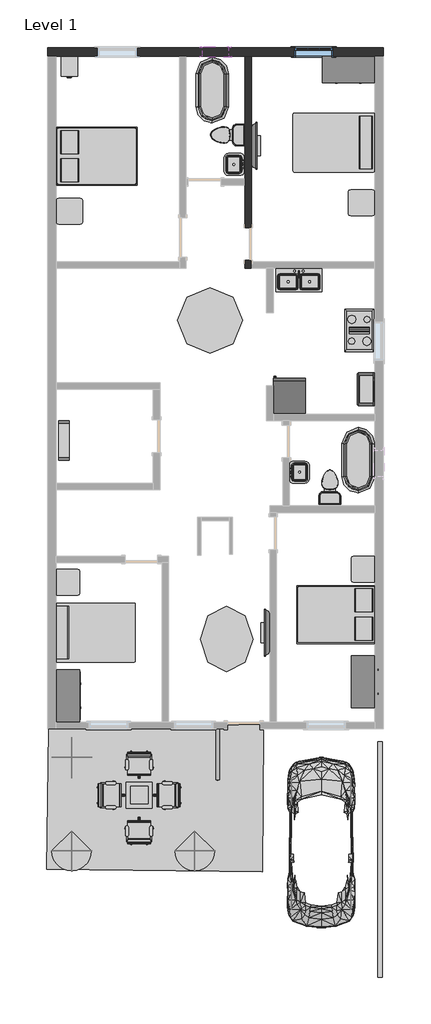
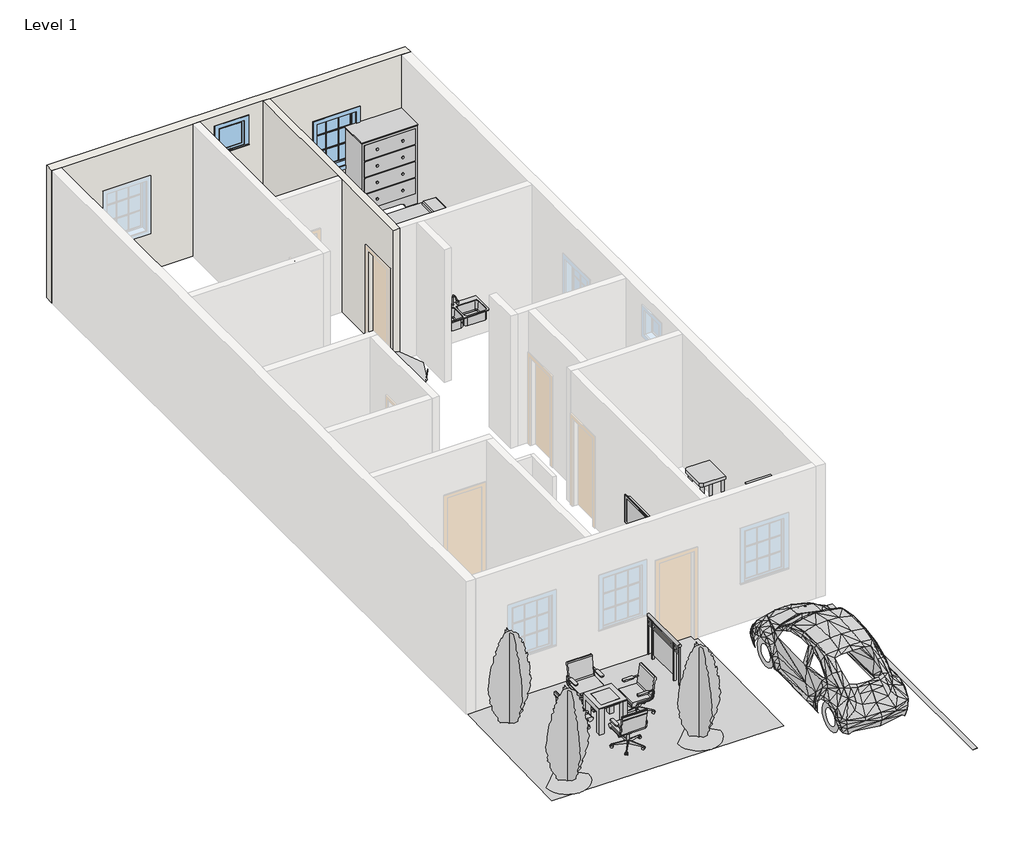
# One storey, part 2 of 2: 22 furniture elements, 7 flow terminals, 6 proxies, 3 geographic elements, 2 walls, 2 windows, 1 railing.
"""IFC4 building model written with IfcOpenShell, lengths in millimetres."""

from ifc_helpers import new_model, si_unit, point, frame, origin, origin_with_axes, place, context, project, spatial, polyline, ellipse_curve, trimmed, outline, extrude, faceted_brep, triangles, transform, mapped, element, save
from ifc_brep_helpers import plane_surface, extruded_surface, advanced_brep
from components import proxy_bb1e6e30, proxy_8a8d5ab2, parking_space_9_x_18_90_deg_b8b21359, rpc_beetle_rpc_beetle_3ce7ba48, proxy_a13a33b2, flow_terminal_a53be723, flow_terminal_62a433f7, toilet_domestic_3d_toilet_domestic_3d_f7549cf7, toilet_domestic_3d_toilet_domestic_3d_183bbd19, flow_terminal_b374fae2, furniture_c8abb964, furniture_0253826f, furniture_552c1472, chair_task_arms_chair_task_arms_fa5a08ef, furniture_9fa109b2, furniture_417d203a, furniture_7a3aaa4f, furniture_b5c51a22, furniture_bbcc68ce, furniture_743965d2, furniture_bcf351fa, rpc_tree_conifer_chinese_juniper_7_1b9786cd, window_29c06734, window_e41d21a6

model = new_model("IFC4")

# Units and contexts
model_context = context("Model", 3, world=origin())
ifc_project = project(units=[si_unit("LENGTHUNIT", "METRE", prefix="MILLI")], contexts=[model_context])

# Site, building, storey
site = spatial("IfcSite", under=ifc_project)
building = spatial("IfcBuilding", under=site)
storey = spatial("IfcBuildingStorey", under=building, Name="Level 1", Elevation=0.0)

# Proxies
placement = place(None, origin())
element("IfcBuildingElementProxy", 1, Name="Building Element Proxy", at=placement, inside=storey, context=model_context, shape_type="Tessellation", body=[
    triangles([(-16242.6911224, -4685.5730095, 0.0), (-16293.4903473, -7924.0733002, 0.0), (-11264.2903473, -7980.080928, 0.0), (-11238.8907349, -4679.2231064, 0.0), (-11238.8907349, -4653.8232033, 0.0), (-11315.0907349, -4552.2230095, 0.0), (-16242.6911224, -4672.8732033, 0.0)], [[2, 1, 7], [1, 2, 3], [7, 1, 6], [4, 6, 1], [5, 6, 4], [4, 1, 3]], closed=False),
])
proxy_shape = proxy_bb1e6e30(model_context)
element("IfcBuildingElementProxy", 2, Name="Cook Top-4 Unit : 36\" x 20\"", ObjectType="Cook Top-4 Unit : 36\" x 20\"", at=placement, inside=storey, context=model_context, shape_type="MappedRepresentation", body=[
    mapped(proxy_shape, transform((-9003.6905738, 4617.1768478, 0.0), x_axis=(0.0, 1.0000000000000009, 0.0), y_axis=(-1.0000000000000009, 0.0, 0.0), z_axis=(0.0, 0.0, 1.0))),
])
proxy_2_shape = proxy_8a8d5ab2(model_context)
element("IfcBuildingElementProxy", 3, Name="Microwave : 30\" x 16\" x 18\"", ObjectType="Microwave : 30\" x 16\" x 18\"", at=placement, inside=storey, context=model_context, shape_type="MappedRepresentation", body=[
    mapped(proxy_2_shape, transform((-9204.3710796, 2745.2839704, 0.0), x_axis=(0.0, 1.0000000000000002, 0.0), y_axis=(-1.0000000000000002, 0.0, 0.0), z_axis=(0.0, 0.0, 1.0))),
])
parking_space_9_x_18_90_deg_shape = parking_space_9_x_18_90_deg_b8b21359(model_context)
element("IfcBuildingElementProxy", 4, Name="Parking Space : 9' x 18' - 90 deg", ObjectType="Parking Space : 9' x 18' - 90 deg", at=placement, inside=storey, context=model_context, shape_type="MappedRepresentation", body=[
    mapped(parking_space_9_x_18_90_deg_shape, transform((-8521.0905738, -10445.0231522, 0.0), x_axis=(-1.0, 0.0, 0.0), y_axis=(0.0, -1.0, 0.0), z_axis=(0.0, 0.0, 1.0))),
])
rpc_beetle_rpc_beetle_shape = rpc_beetle_rpc_beetle_3ce7ba48(model_context)
element("IfcBuildingElementProxy", 5, Name="RPC Beetle : RPC Beetle", ObjectType="RPC Beetle : RPC Beetle", at=placement, inside=storey, context=model_context, shape_type="MappedRepresentation", body=[
    mapped(rpc_beetle_rpc_beetle_shape, transform((-9892.6905738, -8540.0231522, 0.0), x_axis=(1.0, 0.0, 0.0), y_axis=(0.0, 1.0, 0.0), z_axis=(0.0, 0.0, 1.0))),
])
proxy_3_shape = proxy_a13a33b2(model_context)
element("IfcBuildingElementProxy", 6, Name="Refrigerator : 30\" x 32\" RH", ObjectType="Refrigerator : 30\" x 32\" RH", at=placement, inside=storey, context=model_context, shape_type="MappedRepresentation", body=[
    mapped(proxy_3_shape, transform((-10637.2280738, 3079.2778763, 0.0), x_axis=(-1.0000000000000004, 0.0, 0.0), y_axis=(0.0, -1.0000000000000004, 0.0), z_axis=(0.0, 0.0, 1.0))),
])

# Flow terminals
flow_terminal_shape = flow_terminal_a53be723(model_context)
element("IfcFlowTerminal", 7, ObjectType="Sink Kitchen-Double : 42\" x 21\"", at=placement, inside=storey, context=model_context, shape_type="MappedRepresentation", body=[
    mapped(flow_terminal_shape, transform((-10429.0798144, 5783.2314467, 0.0), x_axis=(1.0, 0.0, 0.0), y_axis=(0.0, 1.0, 0.0), z_axis=(0.0, 0.0, 1.0))),
])
flow_terminal_2_shape = flow_terminal_62a433f7(model_context)
element("IfcFlowTerminal", 8, ObjectType="Sink Vanity-Square : 20\" x 18\"", at=placement, inside=storey, context=model_context, shape_type="MappedRepresentation", body=[
    mapped(flow_terminal_2_shape, transform((-11876.2359749, 8493.6660883, 304.8), x_axis=(0.0, -1.0000000000000004, 0.0), y_axis=(1.0000000000000004, 0.0, 0.0), z_axis=(0.0, 0.0, 1.0))),
])
element("IfcFlowTerminal", 9, ObjectType="Sink Vanity-Square : 20\" x 18\"", at=placement, inside=storey, context=model_context, shape_type="MappedRepresentation", body=[
    mapped(flow_terminal_2_shape, transform((-10449.1451727, 1299.4876072, 304.8), x_axis=(0.0, 1.0, 0.0), y_axis=(-1.0, 0.0, 0.0), z_axis=(0.0, 0.0, 1.0))),
])
toilet_domestic_3d_toilet_domestic_3d_shape = toilet_domestic_3d_toilet_domestic_3d_f7549cf7(model_context)
toilet_domestic_3d_toilet_domestic_3d_2_shape = toilet_domestic_3d_toilet_domestic_3d_183bbd19(model_context)
element("IfcFlowTerminal", 10, ObjectType="Toilet-Domestic-3D : Toilet-Domestic-3D", at=placement, inside=storey, context=model_context, shape_type="MappedRepresentation", body=[
    mapped(toilet_domestic_3d_toilet_domestic_3d_shape, transform((-12165.3866012, 9163.7768478, 0.0), x_axis=(0.0, -1.0000000000000002, 0.0), y_axis=(1.0000000000000002, 0.0, 0.0), z_axis=(0.0, 0.0, 1.0))),
    mapped(toilet_domestic_3d_toilet_domestic_3d_2_shape, transform((-12165.3866012, 9163.7768478, 0.0), x_axis=(0.0, -1.0000000000000002, 0.0), y_axis=(1.0000000000000002, 0.0, 0.0), z_axis=(0.0, 0.0, 1.0))),
])
element("IfcFlowTerminal", 11, ObjectType="Toilet-Domestic-3D : Toilet-Domestic-3D", at=placement, inside=storey, context=model_context, shape_type="MappedRepresentation", body=[
    mapped(toilet_domestic_3d_toilet_domestic_3d_shape, transform((-9689.4905738, 1061.1768478, 0.0), x_axis=(-0.9999999999999998, 0.0, 0.0), y_axis=(0.0, -0.9999999999999998, 0.0), z_axis=(0.0, 0.0, 1.0))),
    mapped(toilet_domestic_3d_toilet_domestic_3d_2_shape, transform((-9689.4905738, 1061.1768478, 0.0), x_axis=(-0.9999999999999998, 0.0, 0.0), y_axis=(0.0, -0.9999999999999998, 0.0), z_axis=(0.0, 0.0, 1.0))),
])
flow_terminal_3_shape = flow_terminal_b374fae2(model_context)
element("IfcFlowTerminal", 12, ObjectType="Tub-Free Standing-3D : 30\" x 60\"", at=placement, inside=storey, context=model_context, shape_type="MappedRepresentation", body=[
    mapped(flow_terminal_3_shape, transform((-12432.6905738, 10205.1768478, 0.0), x_axis=(1.0, 0.0, 0.0), y_axis=(0.0, 1.0, 0.0), z_axis=(0.0, 0.0, 1.0))),
])
element("IfcFlowTerminal", 13, ObjectType="Tub-Free Standing-3D : 30\" x 60\"", at=placement, inside=storey, context=model_context, shape_type="MappedRepresentation", body=[
    mapped(flow_terminal_3_shape, transform((-9029.0905738, 1594.5768478, 0.0), x_axis=(1.0, 0.0, 0.0), y_axis=(0.0, 1.0, 0.0), z_axis=(0.0, 0.0, 1.0))),
])

# Furniture
furniture_shape = furniture_c8abb964(model_context)
element("IfcFurniture", 14, ObjectType="Bed-Box : Double 53\" x 74\"", at=placement, inside=storey, context=model_context, shape_type="MappedRepresentation", body=[
    mapped(furniture_shape, transform((-15359.520082, 8329.3243888, 0.0), x_axis=(0.0, 1.0, 0.0), y_axis=(-1.0, 0.0, 0.0), z_axis=(0.0, 0.0, 1.0))),
])
element("IfcFurniture", 15, ObjectType="Bed-Box : Double 53\" x 74\"", at=placement, inside=storey, context=model_context, shape_type="MappedRepresentation", body=[
    mapped(furniture_shape, transform((-9289.9610656, -1660.3706932, 0.0), x_axis=(0.0, -1.0, 0.0), y_axis=(1.0, 0.0, 0.0), z_axis=(0.0, 0.0, 1.0))),
])
furniture_2_shape = furniture_0253826f(model_context)
element("IfcFurniture", 16, ObjectType="Bed-Standard.0001 : Double 54\" x 75\"", at=placement, inside=storey, context=model_context, shape_type="MappedRepresentation", body=[
    mapped(furniture_2_shape, transform((-9554.9954918, 9257.4653724, 0.0), x_axis=(0.0, -1.0000000000000002, 0.0), y_axis=(1.0000000000000002, 0.0, 0.0), z_axis=(0.0, 0.0, 1.0))),
])
element("IfcFurniture", 17, ObjectType="Bed-Standard.0001 : Double 54\" x 75\"", at=placement, inside=storey, context=model_context, shape_type="MappedRepresentation", body=[
    mapped(furniture_2_shape, transform((-15221.4856558, -2690.1116768, 0.0), x_axis=(0.0, 1.0, 0.0), y_axis=(-1.0, 0.0, 0.0), z_axis=(0.0, 0.0, 1.0))),
])
furniture_3_shape = furniture_552c1472(model_context)
element("IfcFurniture", 18, ObjectType="Cabinet-File 3 Drawer.0001 : 15\" x 18\"", at=placement, inside=storey, context=model_context, shape_type="MappedRepresentation", body=[
    mapped(furniture_3_shape, transform((-15632.1941268, 10906.1111479, 0.0), x_axis=(1.0, 0.0, 0.0), y_axis=(0.0, 1.0, 0.0), z_axis=(0.0, 0.0, 1.0))),
])
chair_task_arms_chair_task_arms_shape = chair_task_arms_chair_task_arms_fa5a08ef(model_context)
element("IfcFurniture", 19, ObjectType="Chair-Task Arms : Chair-Task Arms", at=placement, inside=storey, context=model_context, shape_type="MappedRepresentation", body=[
    mapped(chair_task_arms_chair_task_arms_shape, transform((-13993.4997541, -5447.6772506, 0.0), x_axis=(-1.0000000000000004, 0.0, 0.0), y_axis=(0.0, -1.0000000000000004, 0.0), z_axis=(0.0, 0.0, 1.0))),
])
element("IfcFurniture", 20, ObjectType="Chair-Task Arms : Chair-Task Arms", at=placement, inside=storey, context=model_context, shape_type="MappedRepresentation", body=[
    mapped(chair_task_arms_chair_task_arms_shape, transform((-14839.2364754, -6062.2323326, 0.0), x_axis=(0.0, -1.0000000000000007, 0.0), y_axis=(1.0000000000000007, 0.0, 0.0), z_axis=(0.0, 0.0, 1.0))),
])
element("IfcFurniture", 21, ObjectType="Chair-Task Arms : Chair-Task Arms", at=placement, inside=storey, context=model_context, shape_type="MappedRepresentation", body=[
    mapped(chair_task_arms_chair_task_arms_shape, transform((-14275.4813935, -7085.7690539, 0.0), x_axis=(1.0, 0.0, 0.0), y_axis=(0.0, 1.0, 0.0), z_axis=(0.0, 0.0, 1.0))),
])
element("IfcFurniture", 22, ObjectType="Chair-Task Arms : Chair-Task Arms", at=placement, inside=storey, context=model_context, shape_type="MappedRepresentation", body=[
    mapped(chair_task_arms_chair_task_arms_shape, transform((-13429.7446722, -6344.2139719, 0.0), x_axis=(0.0, 1.0000000000000002, 0.0), y_axis=(-1.0000000000000002, 0.0, 0.0), z_axis=(0.0, 0.0, 1.0))),
])
furniture_4_shape = furniture_9fa109b2(model_context)
element("IfcFurniture", 23, ObjectType="Dresser : 48\" x 72\" x 24\"", at=placement, inside=storey, context=model_context, shape_type="MappedRepresentation", body=[
    mapped(furniture_4_shape, transform((-8988.497314, 11050.9398019, 0.0), x_axis=(1.0, 0.0, 0.0), y_axis=(0.0, 1.0, 0.0), z_axis=(0.0, 0.0, 1.0))),
])
element("IfcFurniture", 24, ObjectType="Dresser : 48\" x 72\" x 24\"", at=placement, inside=storey, context=model_context, shape_type="MappedRepresentation", body=[
    mapped(furniture_4_shape, transform((-9252.5535279, -3292.4298924, 0.0), x_axis=(0.0, 1.0, 0.0), y_axis=(-1.0, 0.0, 0.0), z_axis=(0.0, 0.0, 1.0))),
])
element("IfcFurniture", 25, ObjectType="Dresser : 48\" x 72\" x 24\"", at=placement, inside=storey, context=model_context, shape_type="MappedRepresentation", body=[
    mapped(furniture_4_shape, transform((-16186.7535279, -3622.6298924, 0.0), x_axis=(0.0, 1.0, 0.0), y_axis=(-1.0, 0.0, 0.0), z_axis=(0.0, 0.0, 1.0))),
])
furniture_5_shape = furniture_417d203a(model_context)
element("IfcFurniture", 26, ObjectType="Shelving : 36\" x 10\" x 72\"", at=placement, inside=storey, context=model_context, shape_type="MappedRepresentation", body=[
    mapped(furniture_5_shape, transform((-16191.8905738, 2051.7768478, 0.0), x_axis=(0.0, 1.0000000000000002, 0.0), y_axis=(-1.0000000000000002, 0.0, 0.0), z_axis=(0.0, 0.0, 1.0))),
])
furniture_6_shape = furniture_7a3aaa4f(model_context)
element("IfcFurniture", 27, ObjectType="TV - Flat Screen : 42\"", at=placement, inside=storey, context=model_context, shape_type="MappedRepresentation", body=[
    mapped(furniture_6_shape, transform((-11459.7519502, 8913.7213619, 914.4), x_axis=(0.0, 1.0, 0.0), y_axis=(-1.0, 0.0, 0.0), z_axis=(0.0, 0.0, 1.0))),
])
element("IfcFurniture", 28, ObjectType="TV - Flat Screen : 42\"", at=placement, inside=storey, context=model_context, shape_type="MappedRepresentation", body=[
    mapped(furniture_6_shape, transform((-11145.0291975, -2422.5676664, 914.4), x_axis=(0.0, -1.0000000000000004, 0.0), y_axis=(1.0000000000000004, 0.0, 0.0), z_axis=(0.0, 0.0, 1.0))),
])
furniture_7_shape = furniture_b5c51a22(model_context)
element("IfcFurniture", 29, ObjectType="Table-Coffee : 24\" x 24\" x 24\"", at=placement, inside=storey, context=model_context, shape_type="MappedRepresentation", body=[
    mapped(furniture_7_shape, transform((-14152.7563405, -6298.43423, 0.0), x_axis=(1.0, 0.0, 0.0), y_axis=(0.0, 1.0, 0.0), z_axis=(0.0, 0.0, 1.0))),
])
furniture_8_shape = furniture_bbcc68ce(model_context)
element("IfcFurniture", 30, ObjectType="Table-Dining Round w Chairs : 60\" Diameter", at=placement, inside=storey, context=model_context, shape_type="MappedRepresentation", body=[
    mapped(furniture_8_shape, transform((-12587.172541, 5030.6555363, 0.0), x_axis=(1.0, 0.0, 0.0), y_axis=(0.0, 1.0, 0.0), z_axis=(0.0, 0.0, 1.0))),
])
furniture_9_shape = furniture_743965d2(model_context)
element("IfcFurniture", 31, ObjectType="Table-Ellipse : 60\" x 48\"", at=placement, inside=storey, context=model_context, shape_type="MappedRepresentation", body=[
    mapped(furniture_9_shape, transform((-12097.4549283, -2571.0231522, 0.0), x_axis=(0.0, 1.0000000000000002, 0.0), y_axis=(-1.0000000000000002, 0.0, 0.0), z_axis=(0.0, 0.0, 1.0))),
])
furniture_10_shape = furniture_bcf351fa(model_context)
element("IfcFurniture", 32, ObjectType="Table-End : 24\" x 24\"", at=placement, inside=storey, context=model_context, shape_type="MappedRepresentation", body=[
    mapped(furniture_10_shape, transform((-16068.6242041, 7233.3768478, 0.0), x_axis=(1.0, 0.0, 0.0), y_axis=(0.0, 1.0, 0.0), z_axis=(0.0, 0.0, 1.0))),
])
element("IfcFurniture", 33, ObjectType="Table-End : 24\" x 24\"", at=placement, inside=storey, context=model_context, shape_type="MappedRepresentation", body=[
    mapped(furniture_10_shape, transform((-9261.4242041, 7436.5768478, 0.0), x_axis=(1.0, 0.0, 0.0), y_axis=(0.0, 1.0, 0.0), z_axis=(0.0, 0.0, 1.0))),
])
element("IfcFurniture", 34, ObjectType="Table-End : 24\" x 24\"", at=placement, inside=storey, context=model_context, shape_type="MappedRepresentation", body=[
    mapped(furniture_10_shape, transform((-9197.9242041, -1097.8231522, 0.0), x_axis=(1.0, 0.0, 0.0), y_axis=(0.0, 1.0, 0.0), z_axis=(0.0, 0.0, 1.0))),
])
element("IfcFurniture", 35, ObjectType="Table-End : 24\" x 24\"", at=placement, inside=storey, context=model_context, shape_type="MappedRepresentation", body=[
    mapped(furniture_10_shape, transform((-16132.1242041, -1402.6231522, 0.0), x_axis=(1.0, 0.0, 0.0), y_axis=(0.0, 1.0, 0.0), z_axis=(0.0, 0.0, 1.0))),
])

# Geographic elements
rpc_tree_conifer_chinese_juniper_7_shape = rpc_tree_conifer_chinese_juniper_7_1b9786cd(model_context)
element("IfcGeographicElement", 36, ObjectType="RPC Tree - Conifer : Chinese Juniper - 7'", at=placement, inside=storey, context=model_context, shape_type="MappedRepresentation", body=[
    mapped(rpc_tree_conifer_chinese_juniper_7_shape, transform((-15709.4872449, -5314.2231522, 0.0), x_axis=(1.0, 0.0, 0.0), y_axis=(0.0, 1.0, 0.0), z_axis=(0.0, 0.0, 1.0))),
])
element("IfcGeographicElement", 37, ObjectType="RPC Tree - Conifer : Chinese Juniper - 7'", at=placement, inside=storey, context=model_context, shape_type="MappedRepresentation", body=[
    mapped(rpc_tree_conifer_chinese_juniper_7_shape, transform((-15709.4872449, -7498.6231522, 0.0), x_axis=(1.0, 0.0, 0.0), y_axis=(0.0, 1.0, 0.0), z_axis=(0.0, 0.0, 1.0))),
])
element("IfcGeographicElement", 38, ObjectType="RPC Tree - Conifer : Chinese Juniper - 7'", at=placement, inside=storey, context=model_context, shape_type="MappedRepresentation", body=[
    mapped(rpc_tree_conifer_chinese_juniper_7_shape, transform((-12839.2872449, -7498.6231522, 0.0), x_axis=(1.0, 0.0, 0.0), y_axis=(0.0, 1.0, 0.0), z_axis=(0.0, 0.0, 1.0))),
])

# Railing
element("IfcRailing", 39, ObjectType="Glass Panel - Bottom Fill", at=placement, inside=storey, context=model_context, shape_type="SolidModel", body=[
    advanced_brep(
    [(-12267.5905738, -4653.8231522, 914.4), (-12343.7905738, -4653.8231522, 914.4), (-12267.5905738, -5847.6231522, 914.4), (-12343.7905738, -5847.6231522, 914.4)],
    [
        (0, 1, ellipse_curve(frame((-12305.6905738, -4653.8231522, 914.4), z_axis=(0.0, 1.0, 0.0), x_axis=(-1.0, 0.0, 0.0)), 38.1, 28.575)),
        (1, 0, ellipse_curve(frame((-12305.6905738, -4653.8231522, 914.4), z_axis=(0.0, 1.0, 0.0), x_axis=(-1.0, 0.0, 0.0)), 38.1, 28.575)),
        (2, 3, ellipse_curve(frame((-12305.6905738, -5847.6231522, 914.4), z_axis=(0.0, -1.0, 0.0), x_axis=(-1.0, 0.0, 0.0)), 38.1, 28.575)),
        (3, 2, ellipse_curve(frame((-12305.6905738, -5847.6231522, 914.4), z_axis=(0.0, -1.0, 0.0), x_axis=(-1.0, 0.0, 0.0)), 38.1, 28.575)),
        (0, 2),
        (3, 1),
    ],
    [
        plane_surface(frame((-12305.6905738, -4653.8231522, 914.4), z_axis=(0.0, 1.0, 0.0), x_axis=(0.0, 0.0, -1.0))),
        plane_surface(frame((-12305.6905738, -5847.6231522, 914.4), z_axis=(0.0, -1.0, 0.0), x_axis=(0.0, 0.0, -1.0))),
        extruded_surface(trimmed(ellipse_curve(frame((-12305.6905738, -5847.6231522, 914.4), z_axis=(0.0, 1.0, 0.0), x_axis=(-1.0, 0.0, 0.0)), 38.1, 28.575), [point((-12267.5905738, -5847.6231522, 914.4))], [point((-12343.7905738, -5847.6231522, 914.4))], True, "CARTESIAN"), (0.0, 1193.8000000000002, 0.0), 1193.8000000000002),
        extruded_surface(trimmed(ellipse_curve(frame((-12305.6905738, -5847.6231522, 914.4), z_axis=(0.0, 1.0, 0.0), x_axis=(-1.0, 0.0, 0.0)), 38.1, 28.575), [point((-12343.7905738, -5847.6231522, 914.4))], [point((-12267.5905738, -5847.6231522, 914.4))], True, "CARTESIAN"), (0.0, 1193.8000000000002, 0.0), 1193.8000000000002),
    ],
    [
        (0, [[1, 2]]),
        (1, [[3, 4]]),
        (2, [[-1, 5, -4, 6]]),
        (3, [[-2, -6, -3, -5]]),
    ],
),
    extrude(outline(polyline([(-12318.3905738, -4653.8231522), (-12292.9905738, -4653.8231522), (-12292.9905738, -5847.6231522), (-12318.3905738, -5847.6231522), (-12318.3905738, -4653.8231522)])), frame((0.0, 0.0, 800.1), z_axis=(0.0, 0.0, 1.0), x_axis=(1.0, 0.0, 0.0)), (0.0, 0.0, 1.0), 25.4),
    extrude(outline(polyline([(-12318.3905738, -4653.8231522), (-12292.9905738, -4653.8231522), (-12292.9905738, -5847.6231522), (-12318.3905738, -5847.6231522), (-12318.3905738, -4653.8231522)])), frame((0.0, 0.0, 698.5), z_axis=(0.0, 0.0, 1.0), x_axis=(1.0, 0.0, 0.0)), (0.0, 0.0, 1.0), 25.4),
    extrude(outline(polyline([(-12331.0905738, -5650.7731522), (-12280.2905738, -5650.7731522), (-12280.2905738, -5663.4731522), (-12331.0905738, -5663.4731522), (-12331.0905738, -5650.7731522)])), origin_with_axes(), (0.0, 0.0, 1.0), 885.6788223),
    extrude(outline(polyline([(-12299.1554168, -4844.3231522), (-12299.1554168, -5657.1231522), (-12305.5054168, -5657.1231522), (-12305.5054168, -4844.3231522), (-12299.1554168, -4844.3231522)])), frame((0.0, 0.0, 101.6), z_axis=(0.0, 0.0, 1.0), x_axis=(1.0, 0.0, 0.0)), (0.0, 0.0, 1.0), 596.9),
    extrude(outline(polyline([(-12331.0905738, -4837.9731522), (-12280.2905738, -4837.9731522), (-12280.2905738, -4850.6731522), (-12331.0905738, -4850.6731522), (-12331.0905738, -4837.9731522)])), origin_with_axes(), (0.0, 0.0, 1.0), 885.6788223),
    extrude(outline(polyline([(-12315.2155738, -5834.9231522), (-12296.1655738, -5834.9231522), (-12296.1655738, -5853.9731522), (-12315.2155738, -5853.9731522), (-12315.2155738, -5834.9231522)])), origin_with_axes(), (0.0, 0.0, 1.0), 885.6788223),
    extrude(outline(polyline([(-12315.2155738, -4647.4731522), (-12296.1655738, -4647.4731522), (-12296.1655738, -4666.5231522), (-12315.2155738, -4666.5231522), (-12315.2155738, -4647.4731522)])), origin_with_axes(), (0.0, 0.0, 1.0), 885.6788223),
])

# Walls
element("IfcWall", 40, ObjectType="Generic - 8\"", at=placement, inside=storey, context=model_context, shape_type="Brep", body=[
    faceted_brep([(-16268.0905738, 10992.5768478, 0.0), (-16064.8905738, 10992.5768478, 0.0), (-13194.6905738, 10992.5768478, 0.0), (-13042.2905738, 10992.5768478, 0.0), (-11670.6905738, 10992.5768478, 0.0), (-11518.2905738, 10992.5768478, 0.0), (-8648.0905738, 10992.5768478, 0.0), (-8444.8905738, 10992.5768478, 0.0), (-8444.8905738, 10992.5768478, 3048.0), (-8648.0905738, 10992.5768478, 3048.0), (-11518.2905738, 10992.5768478, 3048.0), (-11670.6905738, 10992.5768478, 3048.0), (-13042.2905738, 10992.5768478, 3048.0), (-13194.6905738, 10992.5768478, 3048.0), (-16064.8905738, 10992.5768478, 3048.0), (-16268.0905738, 10992.5768478, 3048.0), (-14185.2905738, 10992.5768478, 2133.6), (-14185.2905738, 10992.5768478, 914.4), (-15099.6905738, 10992.5768478, 914.4), (-15099.6905738, 10992.5768478, 2133.6), (-9613.2905738, 10992.5768478, 2133.6), (-9613.2905738, 10992.5768478, 914.4), (-10527.6905738, 10992.5768478, 914.4), (-10527.6905738, 10992.5768478, 2133.6), (-12661.2905738, 10992.5768478, 2768.6), (-12051.6905738, 10992.5768478, 2768.6), (-12051.6905738, 10992.5768478, 2159.0), (-12661.2905738, 10992.5768478, 2159.0), (-16268.0905738, 11195.7768478, 0.0), (-16268.0905738, 11195.7768478, 3048.0), (-8444.8905738, 11195.7768478, 3048.0), (-8444.8905738, 11195.7768478, 0.0), (-14185.2905738, 11195.7768478, 2133.6), (-15099.6905738, 11195.7768478, 2133.6), (-15099.6905738, 11195.7768478, 914.4), (-14185.2905738, 11195.7768478, 914.4), (-9613.2905738, 11195.7768478, 2133.6), (-10527.6905738, 11195.7768478, 2133.6), (-10527.6905738, 11195.7768478, 914.4), (-9613.2905738, 11195.7768478, 914.4), (-12661.2905738, 11195.7768478, 2768.6), (-12661.2905738, 11195.7768478, 2159.0), (-12051.6905738, 11195.7768478, 2159.0), (-12051.6905738, 11195.7768478, 2768.6)], [[[0, 1, 2, 3, 4, 5, 6, 7, 8, 9, 10, 11, 12, 13, 14, 15], [16, 17, 18, 19], [20, 21, 22, 23], [24, 25, 26, 27]], [[28, 29, 30, 31], [32, 33, 34, 35], [36, 37, 38, 39], [40, 41, 42, 43]], [[7, 6, 5, 4, 3, 2, 1, 0, 28, 31]], [[8, 7, 31, 30]], [[0, 15, 29, 28]], [[17, 16, 32, 35]], [[18, 17, 35, 34]], [[19, 18, 34, 33]], [[16, 19, 33, 32]], [[21, 20, 36, 39]], [[22, 21, 39, 38]], [[23, 22, 38, 37]], [[20, 23, 37, 36]], [[41, 40, 24, 27]], [[42, 41, 27, 26]], [[43, 42, 26, 25]], [[40, 43, 25, 24]], [[15, 14, 13, 12, 11, 10, 9, 8, 30, 29]]]),
])
element("IfcWall", 41, ObjectType="inner wall", at=placement, inside=storey, context=model_context, shape_type="Brep", body=[
    faceted_brep([(-11670.6905738, 6242.7768478, 2032.0), (-11670.6905738, 6242.7768478, 0.0), (-11670.6905738, 6064.9768478, 0.0), (-11670.6905738, 6064.9768478, 3048.0), (-11670.6905738, 7995.3768478, 3048.0), (-11670.6905738, 8147.7768478, 3048.0), (-11670.6905738, 10992.5768478, 3048.0), (-11670.6905738, 10992.5768478, 0.0), (-11670.6905738, 8147.7768478, 0.0), (-11670.6905738, 7995.3768478, 0.0), (-11670.6905738, 7004.7768478, 0.0), (-11670.6905738, 7004.7768478, 2032.0), (-11518.2905738, 6064.9768478, 0.0), (-11518.2905738, 6217.3768478, 0.0), (-11518.2905738, 6242.7768478, 0.0), (-11518.2905738, 6242.7768478, 2032.0), (-11518.2905738, 7004.7768478, 2032.0), (-11518.2905738, 7004.7768478, 0.0), (-11518.2905738, 10992.5768478, 0.0), (-11518.2905738, 10992.5768478, 3048.0), (-11518.2905738, 6217.3768478, 3048.0), (-11518.2905738, 6064.9768478, 3048.0)], [[[0, 1, 2, 3, 4, 5, 6, 7, 8, 9, 10, 11]], [[12, 13, 14, 15, 16, 17, 18, 19, 20, 21]], [[2, 1, 14, 13, 12]], [[10, 9, 8, 7, 18, 17]], [[7, 6, 19, 18]], [[3, 2, 12, 21]], [[15, 14, 1, 0]], [[16, 15, 0, 11]], [[17, 16, 11, 10]], [[6, 5, 4, 3, 21, 20, 19]]]),
])

# Windows
window_shape = window_29c06734(model_context)
element("IfcWindow", 42, ObjectType="Casement 3x3 with Trim : 36\" x 48\"", at=placement, inside=storey, context=model_context, shape_type="MappedRepresentation", body=[
    mapped(window_shape, transform((-10070.4905738, 11094.1768478, 0.0), x_axis=(1.0, 0.0, 0.0), y_axis=(0.0, 1.0, 0.0), z_axis=(0.0, 0.0, 1.0))),
])
window_2_shape = window_e41d21a6(model_context)
element("IfcWindow", 43, ObjectType="Transom with Trim : 24\" x 24\"", at=placement, inside=storey, context=model_context, shape_type="MappedRepresentation", body=[
    mapped(window_2_shape, transform((-12394.5905738, 11094.1768478, 0.0), x_axis=(-1.0, 0.0, 0.0), y_axis=(0.0, -1.0, 0.0), z_axis=(0.0, 0.0, 1.0))),
])

save(model, "model.ifc")

# Revit data of these elements
# Type "Cook Top-4 Unit : 36\" x 20\""
#   Assembly Code = "E1090400"
#   Depth = 2' - 0"
#   Width = 3' - 0"
#   Burner Material = Steel, Chrome Plated
#   Cooktop Material = Steel, Polished
#   Default Elevation = 0
# Type "Microwave : 30\" x 16\" x 18\""
#   Assembly Code = "E1090400"
#   Depth = 1' - 4"
#   Height = 1' - 6"
#   Width = 2' - 6"
#   Microwave Material = Laminate, Ivory, Matte
#   Default Elevation = 0
# Type "Parking Space : 9' x 18' - 90 deg"
#   Angle = 90.00°
#   Parking Length = 18' - 0"
#   Parking Width = 9' - 0"
#   pl = 18' - 0"
#   pw = 9' - 0"
# Type "RPC Beetle : RPC Beetle"
#   built-in parameter 1005195 = "RPC-16-0U6E-L4EG-ENH1-J3KF-SVEL-0TX4-C0"
#   Height = 0
# Type "Refrigerator : 30\" x 32\" RH"
#   Label = "REF."
#   Assembly Code = "E1090400"
#   Depth = 2' - 7 3/4"
#   Handle = 2' - 3"
#   Height = 5' - 10"
#   Rear Clearance = 0' - 2"
#   Top Door Height = 1' - 8"
#   Width = 2' - 5 3/8"
#   Material = Steel, Paint Finish, Ivory, Glossy
#   Default Elevation = 0
# Type "Sink Kitchen-Double : 42\" x 21\""
#   Assembly Code = "D2010410"
#   Counter Height = 3' - 0"
#   Depth = 1' - 9"
#   Width = 3' - 6"
#   Faucet Material = Steel, Polished
#   Sink Material = Steel, Polished
#   Default Elevation = 0
# Type "Sink Vanity-Square : 20\" x 18\""
#   Assembly Code = "D2010400"
#   Counter Height = 2' - 7"
#   Depth = 1' - 6"
#   Width = 1' - 8"
#   Basin Material = Porcelain, Linen
#   Faucet Material = Steel, Polished
#   Default Elevation = 0
# Type "Toilet-Domestic-3D : Toilet-Domestic-3D"
#   Assembly Code = "D2010110"
#   Toilet - Bowl/Basin Material = Porcelain, Linen
#   Toilet - Seat Material = Laminate, Linen, Matte
#   Default Elevation = 0
# Type "Tub-Free Standing-3D : 30\" x 60\""
#   Assembly Code = "D2010110"
#   Height = 1' - 6"
#   Length = 5' - 0"
#   Width = 2' - 6"
#   Tub Material = Porcelain, Ivory
#   Default Elevation = 0
# Type "Bed-Box : Double 53\" x 74\""
#   Assembly Code = "E2020200"
#   Length = 6' - 2"
#   Width = 4' - 5"
#   Frame Material = Birch
#   Mattress Material = Linen, White
#   Default Elevation = 0
# Type "Bed-Standard.0001 : Double 54\" x 75\""
#   Assembly Code = "E2020200"
#   Length = 6' - 3"
#   Width = 4' - 6"
#   Leg Material = Steel, Chrome Plated
#   Mattress Material = Linen, White
#   Default Elevation = 0
# Type "Cabinet-File 3 Drawer.0001 : 15\" x 18\""
#   Assembly Code = "E2020200"
#   Depth = 1' - 6"
#   Height = 3' - 5"
#   Width = 1' - 3"
#   Cabinet Material = Steel, Paint Finish, Ivory, Glossy
#   Handle Material = Steel, Chrome Plated
#   Default Elevation = 0
# Type "Chair-Task Arms : Chair-Task Arms"
#   Assembly Code = "E2020200"
#   Base Material = Plastic, Opaque Black
#   Caster Material = Plastic, Opaque Black
#   Seat/Back Material = Textile - Slate Blue
#   Default Elevation = 0
# Type "Dresser : 48\" x 72\" x 24\""
#   Assembly Code = "E2020200"
#   Depth = 2' - 0"
#   Height = 6' - 0"
#   Width = 4' - 0"
#   Dresser Material = Laminate - Ivory, Glossy
#   Drawer Material = Laminate, Ivory, Matte
#   Knob Material = Cherry
#   Default Elevation = 0
# Type "Shelving : 36\" x 10\" x 72\""
#   Assembly Code = "E2020200"
#   Depth = 0' - 10"
#   Height = 6' - 0"
#   Width = 3' - 0"
#   Shelving Unit Material = Birch
#   Default Elevation = 0
# Type "TV - Flat Screen : 42\""
#   SinAng = 0' - 0.0193"
#   L = 3' - 0.71517"
#   H = 1' - 8.65418"
#   Thickness = 0' - 4.33071"
#   Diagonal = 3' - 6.12598"
#   CosAng = 0' - 0.03431"
#   Stand [instance default] = yes
#   Default Elevation = 0
# Type "Table-Coffee : 24\" x 24\" x 24\""
#   Assembly Code = "E2020200"
#   Height = 2' - 0"
#   Length = 2' - 0"
#   Width = 2' - 0"
#   Top Material = none
#   Frame Material = none
#   Default Elevation = 0
# Type "Table-Dining Round w Chairs : 60\" Diameter"
#   Assembly Code = "E2020200"
#   Radius = 2' - 6"
#   Diameter = 5' - 0"
#   Height = 2' - 6"
#   Chairs = 6
#   Base Material = Pine
#   Top Material = Laminate, Linen, Matte
#   Default Elevation = 0
# Type "Table-Ellipse : 60\" x 48\""
#   Assembly Code = "E2020200"
#   Half Width = 2' - 0"
#   Half Length = 2' - 6"
#   Height = 2' - 6"
#   Length = 5' - 0"
#   Width = 4' - 0"
#   Base Material = Birch
#   Top Material = Birch
#   Default Elevation = 0
# Type "Table-End : 24\" x 24\""
#   Assembly Code = "E2020200"
#   Height = 2' - 6"
#   Length = 2' - 0"
#   Width = 2' - 0"
#   Base Material = Birch
#   Top Material = Laminate, Ivory, Matte
#   Default Elevation = 0
# Type "RPC Tree - Conifer : Chinese Juniper - 7'"
#   built-in parameter 1005198 = "{2, 15},{39, RPC-16-FUM3-UUQ0-UBF0-N000-ST1L-LVER-AU},{1, 0},{1, 0},{2, 13},{1, 8},{5, Color},{1, 0},{1, 0},{3, 0.8},{3, 0.8},{3, 0.8},{1, 8},{7, BBoxMin},{1, 0},{1, 0},{1, 0},{1, 0},{1, 0},{1, 8},{7, BBoxMax},{1, 0},{1, 0},{1, 0},{1, 0},{1, 0},{2, 11},{9, RPCTypeId},{1, 0},{1, 0},{39, RPC-16-FUM3-UUQ0-UBF0-N000-ST1L-LVER-AU},{1, 6},{14, RPCPlantHeight},{1, 0},{1, 0},{1, 7},{2, 11},{7, keyword},{1, 0},{1, 0},{34, :RPCs:Trees [General]:Geometry:RPC},{2, 11},{8, category},{1, 0},{1, 0},{15, Trees [General]},{2, 11},{12, LocalizedUID},{1, 0},{1, 0},{15, Chinese Juniper},{2, 14},{6, Height},{1, 0},{1, 0},{1, 7},{1, 2},{16, Cast Reflections},{1, 0},{1, 0},{1, 0},{1, 2},{12, Cast Shadows},{1, 0},{1, 0},{1, 1},{1, 2},{9, Lock View},{1, 0},{1, 0},{1, 0},{1, 4},{5, ViewC},{1, 0},{1, 0},{1, 0},{21, assetlibrary_base.fbx},{1, 5},"
#   built-in parameter 1005195 = "RPC-16-FUM3-UUQ0-UBF0-N000-ST1L-LVER-AU"
#   Type Comments = "Chinese Juniper"
#   Assembly Code = "G2050500"
#   Height = 7' - 0"
#   Description = (empty or 0)
#   Default Elevation = 0
# Type "Glass Panel - Bottom Fill"
#   Assembly Code = "C2010400"
#   built-in parameter 1008612 = 0.0416667 (stored number, unit not read)
#   built-in parameter 1008611 = 0.0416667 (stored number, unit not read)
#   built-in parameter 1008609 = 0.333333 (stored number, unit not read)
#   built-in parameter 1008604 = 0.166667 (stored number, unit not read)
#   built-in parameter 1008603 = 0.166667 (stored number, unit not read)
#   Railing Height = 3' - 0"
#   built-in parameter 1008630 = 2
#   built-in parameter 1008610 = 2
#   built-in parameter 1008618 = Baluster - Square : 3/4"
# Type "Generic - 8\""
#   Assembly Code = "B2010"
#   Layers, outside or top first: 0' - 8" "Brick, Common" (function 1)
# Type "inner wall"
#   Assembly Code = "B2010"
#   Layers, outside or top first: 0' - 6" "Brick, Common" (function 1)
# Type "Casement 3x3 with Trim : 36\" x 48\""
#   Type Mark = "10"
#   Construction Type Id = "GSP4R"
#   Assembly Code = "B2020100"
#   Analytic Construction = "1/8 in Pilkington single glazing"
#   Visual Light Transmittance = 0.9
#   Solar Heat Gain Coefficient = 0.78
#   Heat Transfer Coefficient (U) = 0.6496 BTU/(h·ft²·°F)
#   Height = 4' - 0"
#   Default Sill Height = 3' - 0"
#   Trim Projection - Ext. = 0' - 0 1/2"
#   Trim Projection - Int. = 0' - 0 3/4"
#   Trim Width - Exterior = 0' - 3 1/2"
#   Trim Width - Interior = 0' - 3 1/2"
#   Width = 3' - 0"
#   Window Inset = 0' - 0 3/4"
#   Define Thermal Properties by = 1
#   Glass Pane Material = Glass
#   Sash Material = Sash
#   Trim Exterior Material = Trim
#   Trim Interior Material = Trim
#   Wall Closure = (empty or 0)
# Type "Transom with Trim : 24\" x 24\""
#   Type Mark = "13"
#   Construction Type Id = "GSP4R"
#   Assembly Code = "B2020100"
#   Analytic Construction = "1/8 in Pilkington single glazing"
#   Visual Light Transmittance = 0.9
#   Solar Heat Gain Coefficient = 0.78
#   Heat Transfer Coefficient (U) = 0.6496 BTU/(h·ft²·°F)
#   Height = 2' - 0"
#   Default Sill Height = 7' - 1"
#   Trim Projection - Ext. = 0' - 0 1/2"
#   Trim Projection - Int. = 0' - 0 3/4"
#   Trim Width - Exterior = 0' - 3 1/2"
#   Trim Width - Interior = 0' - 3 1/2"
#   Width = 2' - 0"
#   Window Inset = 0' - 0 3/4"
#   Define Thermal Properties by = 1
#   Glass Pane Material = Glass
#   Sash Material = Sash
#   Trim Exterior Material = Trim
#   Trim Interior Material = Trim
#   Wall Closure = (empty or 0)
# Element 1 (IfcBuildingElementProxy)
#   Material = none
#   Phase Created = New Construction
# Element 2 (IfcBuildingElementProxy, "Cook Top-4 Unit : 36\" x 20\"")
#   Phase Created = New Construction
#   Materials on its faces: "Steel, Chrome Plated", "Steel, Polished"
# Element 3 (IfcBuildingElementProxy, "Microwave : 30\" x 16\" x 18\"")
#   Phase Created = New Construction
#   Materials on its faces: "Laminate, Ivory, Matte", "Glass"
# Element 4 (IfcBuildingElementProxy, "Parking Space : 9' x 18' - 90 deg")
#   Phase Created = New Construction
#   Materials on its faces: "Parking Stripe"
# Element 5 (IfcBuildingElementProxy, "RPC Beetle : RPC Beetle")
#   Phase Created = New Construction
# Element 6 (IfcBuildingElementProxy, "Refrigerator : 30\" x 32\" RH")
#   Phase Created = New Construction
#   Materials on its faces: "Steel, Paint Finish, Ivory, Glossy", "Steel, Chrome Plated"
# Element 7 (IfcFlowTerminal, "Sink Kitchen-Double : 42\" x 21\"")
#   Mark = "4"
#   Phase Created = New Construction
#   Materials on its faces: "Steel, Polished"
# Element 8 (IfcFlowTerminal, "Sink Vanity-Square : 20\" x 18\"")
#   Mark = "3"
#   Phase Created = New Construction
#   Materials on its faces: "Porcelain, Linen", "Steel, Polished"
# Element 9 (IfcFlowTerminal, "Sink Vanity-Square : 20\" x 18\"")
#   Mark = "7"
#   Phase Created = New Construction
#   Materials on its faces: "Porcelain, Linen", "Steel, Polished"
# Element 10 (IfcFlowTerminal, "Toilet-Domestic-3D : Toilet-Domestic-3D")
#   Mark = "2"
#   Phase Created = New Construction
#   Materials on its faces: "Porcelain, Linen", "Laminate, Linen, Matte"
# Element 11 (IfcFlowTerminal, "Toilet-Domestic-3D : Toilet-Domestic-3D")
#   Mark = "5"
#   Phase Created = New Construction
#   Materials on its faces: "Porcelain, Linen", "Laminate, Linen, Matte"
# Element 12 (IfcFlowTerminal, "Tub-Free Standing-3D : 30\" x 60\"")
#   Mark = "1"
#   Phase Created = New Construction
#   Materials on its faces: "Porcelain, Ivory"
# Element 13 (IfcFlowTerminal, "Tub-Free Standing-3D : 30\" x 60\"")
#   Mark = "6"
#   Phase Created = New Construction
#   Materials on its faces: "Porcelain, Ivory"
# Elements 14, 15 (IfcFurniture, "Bed-Box : Double 53\" x 74\"")
#   Phase Created = New Construction
#   Materials on its faces: "Birch", "Linen, White"
# Elements 16, 17 (IfcFurniture, "Bed-Standard.0001 : Double 54\" x 75\"")
#   Phase Created = New Construction
#   Materials on its faces: "Linen, White", "Steel, Chrome Plated"
# Element 18 (IfcFurniture, "Cabinet-File 3 Drawer.0001 : 15\" x 18\"")
#   Phase Created = New Construction
#   Materials on its faces: "Steel, Chrome Plated", "Steel, Paint Finish, Ivory, Glossy"
# Elements 19, 20, 21, 22 (IfcFurniture, "Chair-Task Arms : Chair-Task Arms")
#   Phase Created = New Construction
#   Materials on its faces: "Plastic, Opaque Black", "Textile - Slate Blue"
# Elements 23, 24, 25 (IfcFurniture, "Dresser : 48\" x 72\" x 24\"")
#   Phase Created = New Construction
#   Materials on its faces: "Laminate, Ivory, Matte", "Cherry", "Laminate - Ivory, Glossy"
# Element 26 (IfcFurniture, "Shelving : 36\" x 10\" x 72\"")
#   Phase Created = New Construction
#   Materials on its faces: "Birch"
# Elements 27, 28 (IfcFurniture, "TV - Flat Screen : 42\"")
#   Stand = yes
#   Phase Created = New Construction
#   Materials on its faces: "TV - Black", "TV - Glass", "TV - Screen"
# Element 29 (IfcFurniture, "Table-Coffee : 24\" x 24\" x 24\"")
#   Phase Created = New Construction
#   Materials on its faces: "Glass - Clear, Grey"
# Element 30 (IfcFurniture, "Table-Dining Round w Chairs : 60\" Diameter")
#   Phase Created = New Construction
#   Materials on its faces: "Pine", "Laminate, Linen, Matte"
# Element 31 (IfcFurniture, "Table-Ellipse : 60\" x 48\"")
#   Phase Created = New Construction
#   Materials on its faces: "Birch"
# Elements 32, 33, 34, 35 (IfcFurniture, "Table-End : 24\" x 24\"")
#   Phase Created = New Construction
#   Materials on its faces: "Laminate, Ivory, Matte", "Birch"
# Elements 36, 37, 38 (IfcGeographicElement, "RPC Tree - Conifer : Chinese Juniper - 7'")
#   Phase Created = New Construction
# Element 39 (IfcRailing, "Glass Panel - Bottom Fill")
#   Phase Created = New Construction
#   Materials on its faces: "Glass"
# Element 40 (IfcWall, "Generic - 8\"")
#   Top Offset = 0' - 0"
#   Base Offset = 0' - 0"
#   Unconnected Height = 10' - 0"
#   wall height = 10' - 0"
#   Phase Created = New Construction
#   Base Constraint = Level 1
#   Materials on its faces: "Brick, Common"
# Element 41 (IfcWall, "inner wall")
#   Top Offset = 0' - 0"
#   Base Offset = 0' - 0"
#   Unconnected Height = 10' - 0"
#   wall height = 10' - 0"
#   Phase Created = New Construction
#   Base Constraint = Level 1
#   Materials on its faces: "Brick, Common"
# Element 42 (IfcWindow, "Casement 3x3 with Trim : 36\" x 48\"")
#   Mark = "2"
#   Phase Created = New Construction
#   Materials on its faces: "Sash", "Glass", "Trim"
# Element 43 (IfcWindow, "Transom with Trim : 24\" x 24\"")
#   Mark = "8"
#   Phase Created = New Construction
#   Materials on its faces: "Sash", "Trim", "Glass"
# Materials
#   "Steel, Chrome Plated": class "Metal", colour RGB 17 17 17, transparency 0, Description = "Chromiuim plated steel", Cost = 0
#   "Steel, Polished": class "Metal", colour RGB 57 57 57, transparency 0, Description = "Polished steel", Cost = 0
#   "Laminate, Ivory, Matte": class "Plastic", colour RGB 247 247 239, transparency 0, Description = "Plastic Laminate - Ivory, Matte", Cost = 0
#   "Steel, Paint Finish, Ivory, Glossy": class "Metal", colour RGB 247 247 239, transparency 0, Description = "Steel, paint finish, ivory, glossy", Cost = 0
#   "Porcelain, Linen": class "Ceramic", colour RGB 249 239 230, transparency 0, Description = "Porcelain, linen", Cost = 0
#   "Laminate, Linen, Matte": class "Plastic", colour RGB 249 239 230, transparency 0, Description = "Plastic Laminate - Linen, Matte", Cost = 0
#   "Porcelain, Ivory": class "Ceramic", colour RGB 247 247 239, transparency 0, Description = "Porcelain, ivory", Cost = 0
#   "Birch": class "Wood", colour RGB 224 178 126, transparency 0, Description = "Betula Alleghaniensis", Cost = 0
#   "Linen, White": class "Textile", colour RGB 247 247 239, transparency 0, Description = "Linen, white", Cost = 0
#   "Plastic, Opaque Black": class "Plastic", colour RGB 0 0 0, transparency 0.7, Description = "Plastic, generic, opaque black", Cost = 0
#   "Textile - Slate Blue": class "Fabric", colour RGB 98 102 118, transparency 0
#   "Laminate - Ivory, Glossy": colour RGB 247 247 239, transparency 0
#   "Cherry": class "Wood", colour RGB 226 177 128, transparency 0, Description = "Prunus Serotina", Cost = 0
#   "Pine": class "Wood", colour RGB 223 192 134, transparency 0, Description = "Pinus Echinata", Cost = 0
#   "Brick, Common": class "Masonry", colour RGB 170 98 104, transparency 0, Description = "Common brick", Cost = 0
#   "Glass": class "Glass", colour RGB 0 128 192, transparency 0.75, Description = "Soda Lime Glass", Cost = 0
#   "Sash": class "Wood", colour RGB 224 178 126, transparency 0
#   "Trim": class "Wood", colour RGB 224 178 126, transparency 0
#   "Parking Stripe": class "Paint", colour RGB 250 250 91, transparency 0
#   "TV - Black": colour RGB 49 49 49, transparency 0
#   "TV - Glass": colour RGB 157 157 157, transparency 0.9
#   "TV - Screen": colour RGB 0 0 0, transparency 0
#   "Glass - Clear, Grey": class "Glass", colour RGB 252 255 255, transparency 0.64
